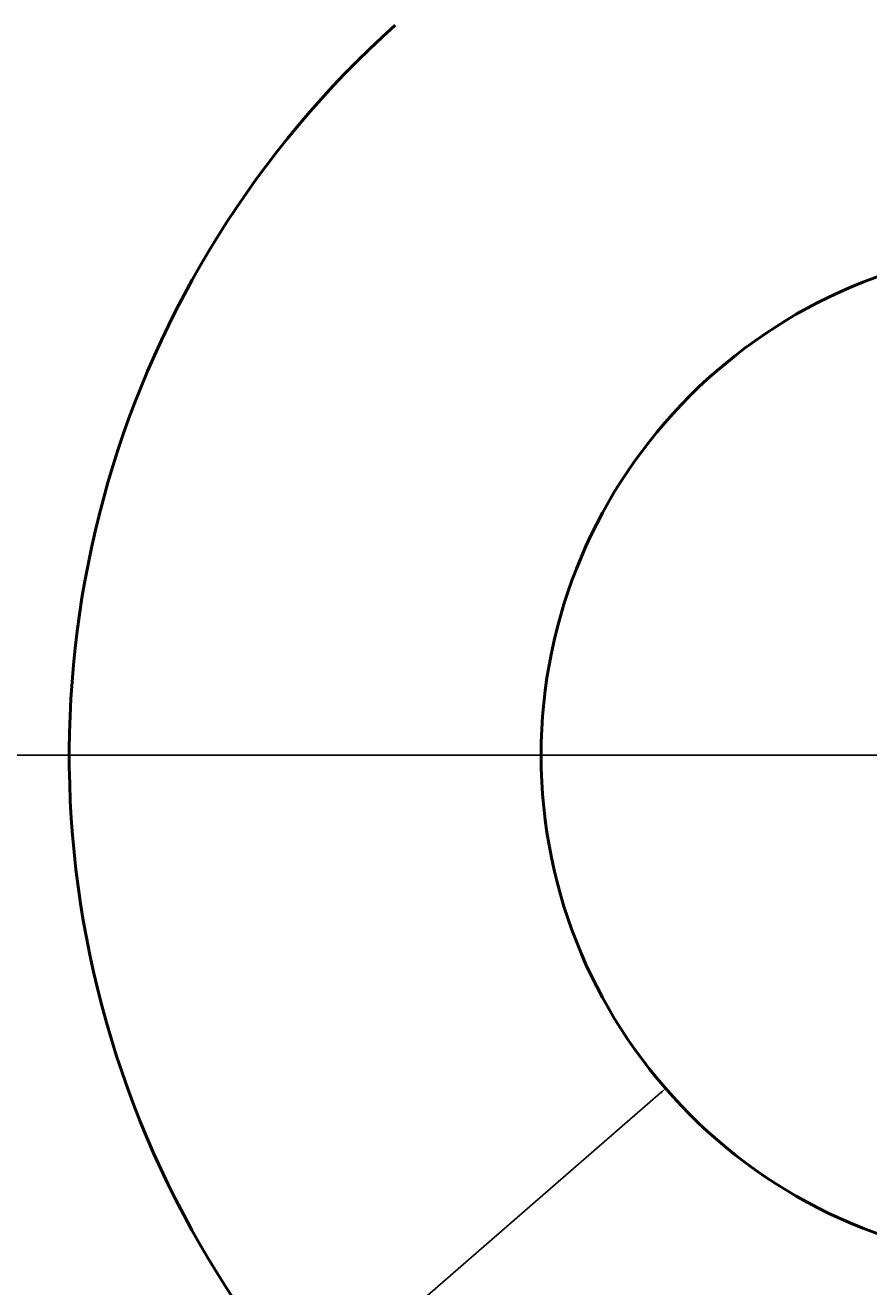
# Model space of a CAD drawing. Units: millimetres. Extents: x -60 to 113, y -37 to 126.
# Tile 3 of 17: x -21 to 2, y -8 to 27. Entities that reach past the tile are written whole.
import ezdxf

# ---------------------------------------------------------------- set-up
doc = ezdxf.new("R2010")
doc.units = ezdxf.units.MM
doc.header["$MEASUREMENT"] = 0
doc.linetypes.add('CENTER2', pattern=[1.125, 0.75, -0.125, 0.125, -0.125])
for name, color, linetype, lineweight in [('M-CNTR', 4, 'CENTER2', 18), ('M-DIMS', 2, 'Continuous', 25), ('M-OUTL', 7, 'Continuous', 50)]:
    doc.layers.add(name, color=color, linetype=linetype, lineweight=lineweight)
doc.styles.get("Standard").update_dxf_attribs({"font": 'arial.ttf'})
doc.dimstyles.get("Standard").update_dxf_attribs({"dimtxt": 0.18, "dimasz": 0.18, "dimexe": 0.18, "dimexo": 0.0625, "dimgap": 0.09, "dimtad": 0, "dimtih": 1, "dimtoh": 1, "dimdec": 4, "dimzin": 0, "dimdsep": 46, "dimtxsty": 'Standard', "dimcen": 0.09, "dimadec": 0, "dimazin": 0, "dimtfac": 1, "dimtdec": 4, "dimtofl": 0, "dimtmove": 0, "dimatfit": 3, "dimfxl": 1, "dimtolj": 1, "dimtzin": 0, "dimarcsym": 0})

# ---------------------------------------------------------------- blocks, each defined once
blk = doc.blocks.new('*U2')
at = {"layer": 'M-CNTR', "color": 0, "transparency": 16777216}
blk.add_line((-27.12, 0), (-5.4, 0), dxfattribs=at)
blk = doc.blocks.new('*D12')
at = {"layer": 'Defpoints', "color": 0, "transparency": 16777216}
for p in [(10.532, 88.533), (-58.719, 6.903), (11.329, 6.903)]:
    blk.add_point(p, dxfattribs=at)
at = {"layer": 'M-DIMS', "color": 0, "lineweight": -2, "transparency": 16777216}
for p, q in [((10.47, 88.533), (-58.899, 88.533)), ((-58.719, 88.353), (-58.719, 48.829)), ((-58.719, 7.083), (-58.719, 46.607)), ((11.267, 6.903), (-58.899, 6.903))]:
    blk.add_line(p, q, dxfattribs=at)
at = {"layer": 'M-DIMS', "color": 0, "transparency": 16777216}
for points in [[(-58.749, 88.353), (-58.689, 88.353), (-58.719, 88.533)], [(-58.749, 7.083), (-58.689, 7.083), (-58.719, 6.903)]]:
    blk.add_solid(points, dxfattribs=at)
at = {"layer": 'M-DIMS', "color": 0, "transparency": 16777216, "insert": (-58.719, 47.718), "char_height": 0.18, "attachment_point": 5}
blk.add_mtext('\\A1;{\\H11.11111x;82}', dxfattribs=at)
blk = doc.blocks.new('*D13')
at = {"layer": 'Defpoints', "color": 0, "transparency": 16777216}
for p in [(37.065, 46.813), (-39.303, 6.903), (7.267, 6.903)]:
    blk.add_point(p, dxfattribs=at)
at = {"layer": 'M-DIMS', "color": 0, "lineweight": -2, "transparency": 16777216}
for p, q in [((37.002, 46.813), (-39.483, 46.813)), ((-39.303, 46.633), (-39.303, 27.969)), ((-39.303, 7.083), (-39.303, 25.747)), ((7.204, 6.903), (-39.483, 6.903))]:
    blk.add_line(p, q, dxfattribs=at)
at = {"layer": 'M-DIMS', "color": 0, "transparency": 16777216}
for points in [[(-39.333, 46.633), (-39.273, 46.633), (-39.303, 46.813)], [(-39.333, 7.083), (-39.273, 7.083), (-39.303, 6.903)]]:
    blk.add_solid(points, dxfattribs=at)
at = {"layer": 'M-DIMS', "color": 0, "transparency": 16777216, "insert": (-39.303, 26.858), "char_height": 0.18, "attachment_point": 5}
blk.add_mtext('\\A1;{\\H11.11111x;40}', dxfattribs=at)
blk = doc.blocks.new('*D15')
at = {"layer": 'Defpoints', "color": 0, "transparency": 16777216}
for p in [(17.836, 16.083), (-3.303, -2.278)]:
    blk.add_point(p, dxfattribs=at)
at = {"layer": 'M-DIMS', "color": 0, "lineweight": -2, "transparency": 16777216}
for p, q in [((7.267, 6.813), (7.267, 6.993)), ((7.177, 6.903), (7.357, 6.903)), ((-20.464, -17.184), (-3.439, -2.396)), ((-20.644, -17.184), (-20.464, -17.184))]:
    blk.add_line(p, q, dxfattribs=at)
at = {"layer": 'M-DIMS', "color": 0, "transparency": 16777216}
blk.add_solid([(-3.459, -2.373), (-3.419, -2.419), (-3.303, -2.278)], dxfattribs=at)
at = {"layer": 'M-DIMS', "color": 0, "transparency": 16777216, "insert": (-24.497, -17.184), "char_height": 0.18, "attachment_point": 5}
blk.add_mtext('\\A1;{\\H11.11111x;3-%%C28}', dxfattribs=at)
blk = doc.blocks.new('HOLE-D28')
blk.add_circle((14, 14), 14)

msp = doc.modelspace()

# ---------------------------------------------------------------- linework, layer by layer
at = {"layer": 'M-OUTL'}
msp.add_arc((7.26659, 6.9027), 27, 131.866655, 323.73509, dxfattribs=at)

# ---------------------------------------------------------------- block references
at = {"layer": 'M-CNTR'}
msp.add_blockref('*U2', (7.26659, 6.9027), dxfattribs=at)
at = {"layer": 'M-OUTL'}
msp.add_blockref('HOLE-D28', (-6.733, -7.097), dxfattribs=at)

# ---------------------------------------------------------------- dimensions: what is measured, and where the dimension line sits
at = {"layer": 'M-DIMS'}
for base, p1, p2, text, picture, middle in [((-58.71857, 6.9027), (10.53227, 88.53289), (11.32938, 6.9027), '{\\H11.11111x;82}', '*D12', (-58.71857, 47.71779)), ((-39.30316, 6.9027), (37.06463, 46.81263), (7.26659, 6.9027), '{\\H11.11111x;40}', '*D13', (-39.30316, 26.85766))]:
    dim = msp.add_linear_dim(base=base, p1=p1, p2=p2, angle=90, text=text, dimstyle='Standard', override={"dimclrd": 0, "dimclre": 0, "dimclrt": 0}, dxfattribs=at)
    dim.commit()
    dim.dimension.update_dxf_attribs({"geometry": picture, "text_midpoint": middle})
dim = msp.add_diameter_dim_2p(p1=(17.83613, 16.08337), p2=(-3.30296, -2.27798), text='{\\H11.11111x;3-%%C28}', dimstyle='Standard', override={"dimclrd": 0, "dimclre": 0, "dimclrt": 0}, dxfattribs=at)
dim.commit()
dim.dimension.update_dxf_attribs({"geometry": '*D15', "text_midpoint": (-24.49681, -17.18418), "dimtype": 163})

doc.saveas('drawing.dxf')
